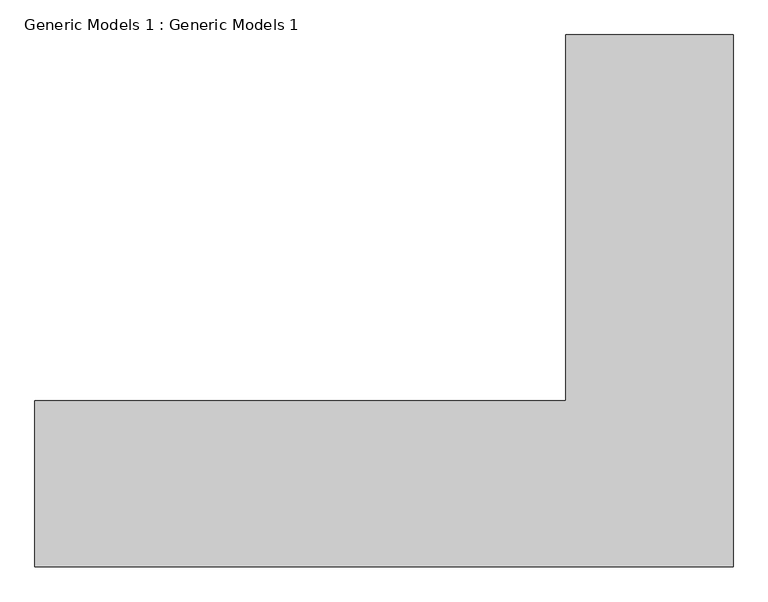
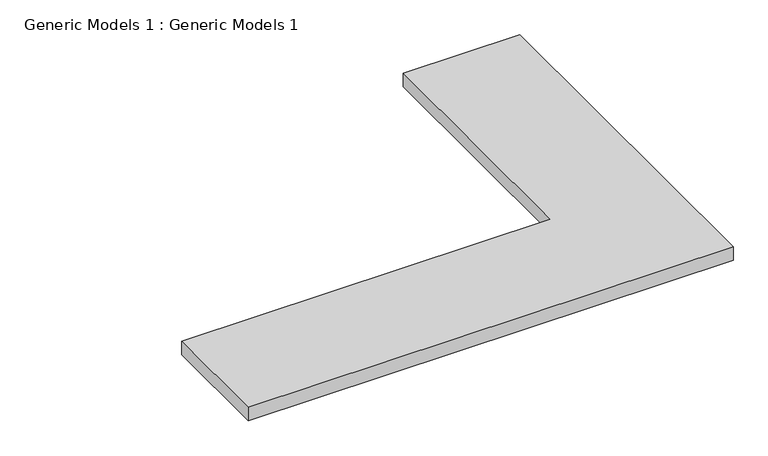
"""IFC4 building model written with IfcOpenShell, lengths in millimetres: proxy geometry, Generic Models 1 : Generic Models 1."""

from ifc_helpers import new_model, si_unit, frame, origin, place, context, project, spatial, polyline, outline, extrude, source, transform, mapped, element, save


def generic_models_1_generic_models_1_a00969f3(model_context):
    return source(origin(), model_context, "Body", "SweptSolid", [
        extrude(outline(polyline([(-5884.523883, 2580.8820885), (-5884.523883, 3940.2580989), (-5262.223883, 3940.2580989), (-5262.223883, 2580.8820885), (-5262.223883, 1964.8606314), (-7855.563883, 1964.8606314), (-7855.563883, 2580.8820885), (-5884.523883, 2580.8820885)])), frame((0.0, 0.0, 1219.2), z_axis=(0.0, 0.0, 1.0), x_axis=(1.0, 0.0, 0.0)), (0.0, 0.0, 1.0), 76.2),
    ])


if __name__ == "__main__":
    model = new_model("IFC4")
    model_context = context("Model", 3, world=origin())
    ifc_project = project(units=[si_unit("LENGTHUNIT", "METRE", prefix="MILLI")], contexts=[model_context])
    site = spatial("IfcSite", under=ifc_project)
    building = spatial("IfcBuilding", under=site)
    placement = place(None, origin())
    generic_models_1_generic_models_1_shape = generic_models_1_generic_models_1_a00969f3(model_context)
    element("IfcBuildingElementProxy", 1, Name="Generic Models 1 : Generic Models 1", ObjectType="Generic Models 1 : Generic Models 1", at=placement, inside=building, context=model_context, shape_type="MappedRepresentation", body=[
        mapped(generic_models_1_generic_models_1_shape, transform((0.0, 0.0, 0.0), x_axis=(1.0, 0.0, 0.0), y_axis=(0.0, 1.0, 0.0), z_axis=(0.0, 0.0, 1.0))),
    ])
    save(model, "model.ifc")

# Revit data of these elements
# Element 1 (IfcBuildingElementProxy, "Generic Models 1 : Generic Models 1")
#   Materials on its faces: "Concrete, Precast"
# Materials
#   "Concrete, Precast": class "Concrete", colour RGB 192 192 192, transparency 0, Description = "Precast concrete", Cost = 0
